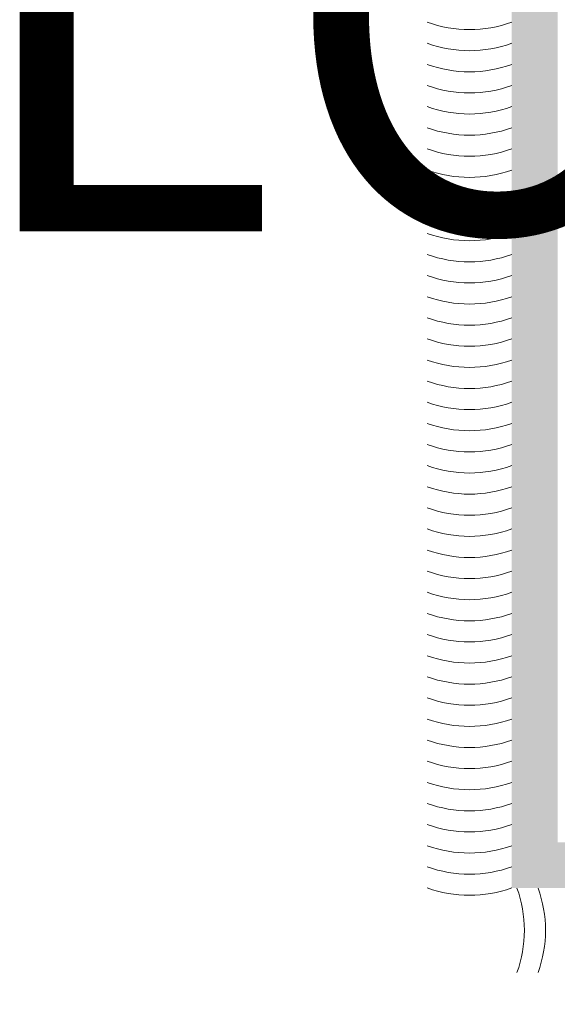
# Model space of a CAD drawing. Units: inches. Extents: x 844 to 2234, y 346 to 1084.
# Tile 68 of 93: x 1989.98 to 1997.48, y 687.63 to 701.36. Entities that reach past the tile are written whole.
import ezdxf

# ---------------------------------------------------------------- set-up
doc = ezdxf.new("R2010")
doc.units = ezdxf.units.IN
doc.header["$MEASUREMENT"] = 0
for name, color, linetype, lineweight in [('A-ANNO-DIMS', 2, 'Continuous', 18), ('furniture', 8, 'Continuous', 18), ('RA-AP-01$0$INT', 35, 'Continuous', 5)]:
    doc.layers.add(name, color=color, linetype=linetype, lineweight=lineweight)
doc.layers.add('RA-AP-01$0$FURN', color=3, linetype='Continuous')
doc.styles.get("Standard").update_dxf_attribs({"font": 'arial.ttf'})
doc.dimstyles.get("Standard").update_dxf_attribs({"dimtxt": 6, "dimasz": 3, "dimexe": 0.18, "dimexo": 0.0625, "dimgap": 0.09, "dimtad": 0, "dimtih": 1, "dimtoh": 1, "dimdec": 1, "dimzin": 0, "dimdsep": 46, "dimlunit": 3, "dimtxsty": 'Standard', "dimblk": 'ARCHTICK', "dimcen": 0.09, "dimadec": 0, "dimazin": 0, "dimtfac": 1, "dimtdec": 1, "dimtofl": 0, "dimtmove": 0, "dimatfit": 3, "dimfxl": 1, "dimtolj": 1, "dimtzin": 0, "dimarcsym": 0})

# ---------------------------------------------------------------- blocks, each defined once
blk = doc.blocks.new('A$C18D01794')
at = {"layer": 'RA-AP-01$0$INT'}
h = blk.add_hatch(color=256, dxfattribs=at)
h.paths.add_polyline_path([(4.3552, -6.1567), (4.3552, -8.0567), (5.4552, -8.0567), (5.4552, -6.1567)])
h.paths.add_polyline_path([(4.4052, -8.0067), (4.4052, -6.2067), (5.4052, -6.2067), (5.4052, -8.0067)], flags=16)
for centre, start, end in [((5.5548, -6.1105), 160.2038, 199.7962), ((5.5779, -6.1105), 160.2038, 199.7962), ((5.5014, -6.2852), 70.2038, 109.7962), ((5.5014, -6.3083), 70.2038, 109.7962), ((5.5014, -6.3314), 70.2038, 109.7962), ((5.5014, -6.3545), 70.2038, 109.7962), ((5.5014, -6.3776), 70.2038, 109.7962), ((5.5014, -6.4007), 70.2038, 109.7962), ((5.5014, -6.4238), 70.2038, 109.7962), ((5.5014, -6.4469), 70.2038, 109.7962), ((5.5014, -6.47), 70.2038, 109.7962), ((5.5014, -6.4931), 70.2038, 109.7962), ((5.5014, -6.5162), 70.2038, 109.7962), ((5.5014, -6.5393), 70.2038, 109.7962), ((5.5014, -6.5624), 70.2038, 109.7962), ((5.5014, -6.5855), 70.2038, 109.7962), ((5.5014, -6.6086), 70.2038, 109.7962), ((5.5014, -6.6317), 70.2038, 109.7962), ((5.5014, -6.6548), 70.2038, 109.7962), ((5.5014, -6.6779), 70.2038, 109.7962), ((5.5014, -6.701), 70.2038, 109.7962), ((5.5014, -6.7241), 70.2038, 109.7962), ((5.5014, -6.7472), 70.2038, 109.7962), ((5.5014, -6.7703), 70.2038, 109.7962), ((5.5014, -6.7934), 70.2038, 109.7962), ((5.5014, -6.7934), 70.2038, 109.7962), ((5.5014, -6.8165), 70.2038, 109.7962), ((5.5014, -6.8396), 70.2038, 109.7962), ((5.5014, -6.8627), 70.2038, 109.7962), ((5.5014, -6.8858), 70.2038, 109.7962), ((5.5014, -6.9089), 70.2038, 109.7962), ((5.5014, -6.932), 70.2038, 109.7962), ((5.5014, -6.9551), 70.2038, 109.7962), ((5.5014, -6.9782), 70.2038, 109.7962), ((5.5014, -7.0013), 70.2038, 109.7962), ((5.5014, -7.0244), 70.2038, 109.7962), ((5.5014, -7.0475), 70.2038, 109.7962), ((5.5014, -7.0706), 70.2038, 109.7962), ((5.5014, -7.0937), 70.2038, 109.7962), ((5.5014, -7.1168), 70.2038, 109.7962), ((5.5014, -7.1399), 70.2038, 109.7962), ((5.5014, -7.163), 70.2038, 109.7962), ((5.5014, -7.1861), 70.2038, 109.7962), ((5.5014, -7.2092), 70.2038, 109.7962), ((5.5014, -7.2323), 70.2038, 109.7962)]:
    blk.add_arc(centre, 0.1364, start, end, dxfattribs=at)
blk = doc.blocks.new('A$C5D2F253E')
at = {"layer": 'RA-AP-01$0$FURN', "xscale": -0.7999999999883585, "yscale": 0.7999999999883585, "zscale": 0.8, "rotation": 90}
blk.add_blockref('A$C18D01794', (-5.68776, 4.75792), dxfattribs=at)
blk = doc.blocks.new('_ArchTick')
at = {"color": 0, "linetype": 'ByBlock', "const_width": 0.15}
blk.add_lwpolyline([(-0.5, -0.5), (0.5, 0.5)], dxfattribs=at)
blk = doc.blocks.new('*D121')
at = {"layer": 'A-ANNO-DIMS', "color": 0, "lineweight": -2, "transparency": 16777216}
for p, q in [((2030.272, 734.263), (2040.245, 734.263)), ((2040.065, 734.263), (2040.065, 704.604)), ((2040.065, 668.557), (2040.065, 698.216)), ((2030.272, 668.557), (2040.245, 668.557))]:
    blk.add_line(p, q, dxfattribs=at)
at = {"layer": 'Defpoints', "color": 0, "transparency": 16777216}
for p in [(2030.209, 734.263), (2040.065, 734.263), (2030.209, 668.557)]:
    blk.add_point(p, dxfattribs=at)
at = {"layer": 'A-ANNO-DIMS', "color": 0, "lineweight": -2, "transparency": 16777216, "xscale": 3, "yscale": 3, "zscale": 3}
for p, rotation in [((2040.065, 734.263), 90), ((2040.065, 668.557), 270)]:
    blk.add_blockref('_ArchTick', p, dxfattribs=dict(at, rotation=rotation))
at = {"layer": 'A-ANNO-DIMS', "color": 0, "transparency": 16777216, "insert": (2040.065, 701.41), "char_height": 6, "attachment_point": 5}
blk.add_mtext('\\A1;LOUNGE SET 5\'-5 1/2" TYP.', dxfattribs=at)

msp = doc.modelspace()

# ---------------------------------------------------------------- block references
at = {"layer": 'furniture', "xscale": -15.94108302203742, "yscale": 15.94108302203742, "zscale": 15.94108302203742, "rotation": 270}
msp.add_blockref('A$C5D2F253E', (1990.567, 701.403), dxfattribs=at)

# ---------------------------------------------------------------- dimensions: what is measured, and where the dimension line sits
at = {"layer": 'A-ANNO-DIMS'}
dim = msp.add_linear_dim(base=(2040.065, 734.263), p1=(2030.209, 668.557), p2=(2030.209, 734.263), angle=90, text='LOUNGE SET <> TYP.', dimstyle='Standard', override={"dimdec": 1, "dimlfac": 1, "dimrnd": 0, "dimzin": 1, "dimdsep": 46, "dimlunit": 4, "dimfrac": 2}, dxfattribs=at)
dim.commit()
dim.dimension.update_dxf_attribs({"geometry": '*D121', "text_midpoint": (2040.065, 701.41)})

doc.saveas('drawing.dxf')
